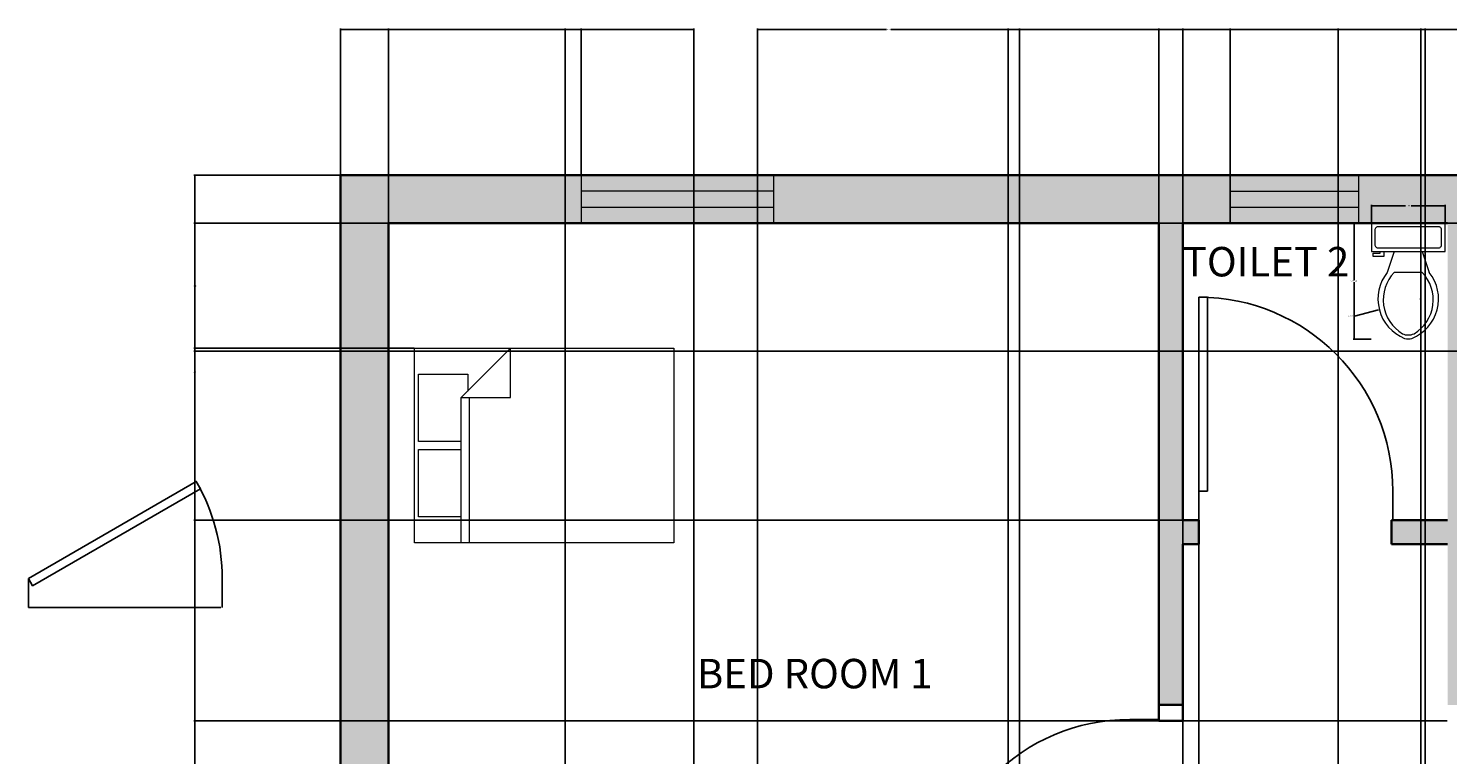
# Model space of a CAD drawing. Units: inches. Extents: x 1839 to 2285, y 722 to 1311.
# Tile 6 of 7: x 1839 to 2105, y 1175 to 1311. Entities that reach past the tile are written whole.
import ezdxf

# ---------------------------------------------------------------- set-up
doc = ezdxf.new("R2010")
doc.units = ezdxf.units.IN
for name, color, linetype, lineweight in [('A-ANNO-DIMS', 2, 'Continuous', 18), ('A-AREA-IDEN', 7, 'Continuous', 18), ('A-DOOR', 3, 'Continuous', 25), ('A-FLOR-FIXT', 9, 'Continuous', 18), ('A-FURN', 8, 'Continuous', 18), ('A-GLAZ', 4, 'Continuous', 18), ('A-GLAZ-PATT', 9, 'Continuous', 13), ('A-WALL', 7, 'Continuous', 35)]:
    doc.layers.add(name, color=color, linetype=linetype, lineweight=lineweight)
doc.layers.add('A-WALL-PATT', color=18, linetype='Continuous', lineweight=13, true_color=0x000000)
doc.styles.get("Standard").update_dxf_attribs({"font": 'arial.ttf'})
doc.dimstyles.get("Standard").update_dxf_attribs({"dimtxt": 0.18, "dimasz": 0.18, "dimexe": 0.18, "dimexo": 0.0625, "dimgap": 0.09, "dimtad": 0, "dimtih": 1, "dimtoh": 1, "dimdec": 4, "dimzin": 0, "dimdsep": 46, "dimtxsty": 'Standard', "dimcen": 0.09, "dimadec": 0, "dimazin": 0, "dimtfac": 1, "dimtdec": 4, "dimtofl": 0, "dimtmove": 0, "dimatfit": 3, "dimfxl": 1, "dimtolj": 1, "dimtzin": 0, "dimarcsym": 0})

# ---------------------------------------------------------------- blocks, each defined once
blk = doc.blocks.new('*U2')
for p, q in [((0, 0), (0, -6)), ((40, 0), (40, -6))]:
    blk.add_line(p, q)
blk.add_lwpolyline([(0, 0), (34.64, 20), (35.52, 18.48), (0.87, -1.52)], close=True)
blk.add_arc((0, 0), 40, 0, 30)
blk = doc.blocks.new('*U4')
for p, q in [((0, 0), (0, -6)), ((40, 0), (40, -6))]:
    blk.add_line(p, q)
blk.add_lwpolyline([(0, 0), (0, 40), (1.75, 40), (1.75, 0)], close=True)
blk.add_arc((0, 0), 40, 0, 90)
blk = doc.blocks.new('Toilet - top')
for p, q in [((9.5, -6), (9.5, -2)), ((-8, -8.5), (-8, -8)), ((-7, -8), (-7, -9.5)), ((-4, -8), (-6, -14)), ((4, -8), (6, -14)), ((-10, -8.5), (-8, -8.5)), ((-10, -9.5), (-10, -8.5)), ((-7, -9.5), (-10, -9.5)), ((4, -14), (-4, -14))]:
    blk.add_line(p, q)
blk.add_lwpolyline([(10.5, -8), (10.5, 0), (-10.5, 0), (-10.5, -8)], close=True)
for points in [[(-9.5, -2), (-9.5, -6)], [(8.5, -1), (-8.5, -1)], [(-8.5, -7), (8.5, -7)]]:
    blk.add_lwpolyline(points)
for centre, radius, start, end in [((-8.62, -1.88), 0.884, 81.8699, 188.1301), ((8.62, -1.88), 0.884, 351.8699, 98.1301), ((-8.62, -6.12), 0.884, 171.8699, 278.1301), ((8.62, -6.12), 0.884, 261.8699, 8.1301), ((3.52, -21.58), 12.17, 141.4691, 247.9714), ((4.2, -21.82), 11.33, 136.3677, 238.9468), ((-3.52, -21.58), 12.17, 292.0284, 38.5307), ((-4.2, -21.82), 11.33, 301.053, 43.6321), ((0, -27.88), 4, 245.7318, 294.2682), ((0, -29), 4, 254.8605, 285.1395)]:
    blk.add_arc(centre, radius, start, end)
blk = doc.blocks.new('Bed - Queen')
for p, q in [((0, -80.00003), (0, 0)), ((0, 0), (59.99999, 0)), ((59.99999, 0), (59.99999, -80.00003)), ((7.99999, -1.2), (28.79998, -1.2)), ((7.99999, -14.4), (7.99999, -1.2)), ((28.79998, -1.2), (28.79998, -14.4)), ((31.19999, -1.2), (51.99999, -1.2)), ((31.19999, -14.4), (31.19999, -1.2)), ((51.99999, -1.2), (51.99999, -16.4)), ((0, -14.4), (44.8, -14.4)), ((44.8, -16.8), (0, -16.8)), ((59.99999, -29.6), (44.8, -14.4)), ((44.8, -14.4), (44.8, -29.6)), ((51.99999, -16.4), (46.79936, -16.4)), ((44.8, -29.6), (59.99999, -29.6)), ((59.99999, -80.00003), (0, -80.00003))]:
    blk.add_line(p, q)
blk = doc.blocks.new('WIN-36x9')
for p, q in [((0, 9), (0, 0)), ((36, 9), (0, 9)), ((36, 0), (36, 9)), ((36, 6), (0, 6)), ((0, 3), (36, 3)), ((0, 0), (36, 0))]:
    blk.add_line(p, q)
blk = doc.blocks.new('WIN-24x9')
for p, q in [((3, 0), (3, 24)), ((6, 0), (6, 24))]:
    blk.add_line(p, q)
blk.add_lwpolyline([(0, 24), (0, 0), (9, 0), (9, 24)], close=True)
blk = doc.blocks.new('*D23')
at = {"layer": 'A-ANNO-DIMS', "color": 0, "lineweight": -2, "transparency": 16777216}
for p, q in [((2090.38, 1274.33), (2087.01, 1274.33)), ((2087.19, 1274.15), (2087.19, 1263.69)), ((2087.19, 1252.87), (2087.19, 1263.33)), ((2090.38, 1252.69), (2087.01, 1252.69))]:
    blk.add_line(p, q, dxfattribs=at)
at = {"layer": 'A-ANNO-DIMS', "color": 0, "transparency": 16777216}
for points in [[(2087.16, 1274.15), (2087.22, 1274.15), (2087.19, 1274.33)], [(2087.16, 1252.87), (2087.22, 1252.87), (2087.19, 1252.69)]]:
    blk.add_solid(points, dxfattribs=at)
at = {"layer": 'Defpoints', "color": 0, "transparency": 16777216}
for p in [(2087.19, 1274.33), (2090.44, 1274.33), (2090.44, 1252.69)]:
    blk.add_point(p, dxfattribs=at)
at = {"layer": 'A-ANNO-DIMS', "color": 0, "transparency": 16777216, "insert": (2087.19, 1263.51), "char_height": 0.18, "attachment_point": 5}
blk.add_mtext('\\A1;WC 22 TYP.', dxfattribs=at)
blk = doc.blocks.new('*D24')
at = {"layer": 'A-ANNO-DIMS', "color": 0, "lineweight": -2, "transparency": 16777216}
for p, q in [((2090.44, 1274.39), (2090.44, 1277.76)), ((2090.62, 1277.58), (2096.8, 1277.58)), ((2104.01, 1277.58), (2097.84, 1277.58)), ((2104.19, 1274.39), (2104.19, 1277.76))]:
    blk.add_line(p, q, dxfattribs=at)
at = {"layer": 'A-ANNO-DIMS', "color": 0, "transparency": 16777216}
for points in [[(2090.62, 1277.61), (2090.62, 1277.55), (2090.44, 1277.58)], [(2104.01, 1277.61), (2104.01, 1277.55), (2104.19, 1277.58)]]:
    blk.add_solid(points, dxfattribs=at)
at = {"layer": 'Defpoints', "color": 0, "transparency": 16777216}
for p in [(2104.19, 1277.58), (2090.44, 1274.33), (2104.19, 1274.33)]:
    blk.add_point(p, dxfattribs=at)
at = {"layer": 'A-ANNO-DIMS', "color": 0, "transparency": 16777216, "insert": (2097.32, 1277.58), "char_height": 0.18, "attachment_point": 5}
blk.add_mtext('\\A1;14 TYP.', dxfattribs=at)
blk = doc.blocks.new('*D42')
at = {"layer": 'A-ANNO-DIMS', "color": 0, "lineweight": -2, "transparency": 16777216}
for p, q in [((1897.61, 1283.33), (1870.25, 1283.33)), ((1870.43, 1283.15), (1870.43, 1043.51)), ((1870.43, 803.51), (1870.43, 1043.15)), ((1897.61, 803.33), (1870.25, 803.33))]:
    blk.add_line(p, q, dxfattribs=at)
at = {"layer": 'A-ANNO-DIMS', "color": 0, "transparency": 16777216}
for points in [[(1870.4, 1283.15), (1870.46, 1283.15), (1870.43, 1283.33)], [(1870.4, 803.51), (1870.46, 803.51), (1870.43, 803.33)]]:
    blk.add_solid(points, dxfattribs=at)
at = {"layer": 'Defpoints', "color": 0, "transparency": 16777216}
for p in [(1870.43, 1283.33), (1897.68, 1283.33), (1897.68, 803.33)]:
    blk.add_point(p, dxfattribs=at)
at = {"layer": 'A-ANNO-DIMS', "color": 0, "transparency": 16777216, "insert": (1870.43, 1043.33), "char_height": 0.18, "attachment_point": 5}
blk.add_mtext('\\A1;480', dxfattribs=at)
blk = doc.blocks.new('*D47')
at = {"layer": 'A-ANNO-DIMS', "color": 0, "lineweight": -2, "transparency": 16777216}
for p, q in [((2055.11, 1274.33), (1870.25, 1274.33)), ((1870.43, 1274.15), (1870.43, 1246.76)), ((1870.43, 1219.01), (1870.43, 1246.4)), ((2055.11, 1218.83), (1870.25, 1218.83))]:
    blk.add_line(p, q, dxfattribs=at)
at = {"layer": 'A-ANNO-DIMS', "color": 0, "transparency": 16777216}
for points in [[(1870.4, 1274.15), (1870.46, 1274.15), (1870.43, 1274.33)], [(1870.4, 1219.01), (1870.46, 1219.01), (1870.43, 1218.83)]]:
    blk.add_solid(points, dxfattribs=at)
at = {"layer": 'Defpoints', "color": 0, "transparency": 16777216}
for p in [(1870.43, 1274.33), (2055.18, 1274.33), (2055.18, 1218.83)]:
    blk.add_point(p, dxfattribs=at)
at = {"layer": 'A-ANNO-DIMS', "color": 0, "transparency": 16777216, "insert": (1870.43, 1246.58), "char_height": 0.18, "attachment_point": 5}
blk.add_mtext('\\A1;55.5', dxfattribs=at)
blk = doc.blocks.new('*D53')
at = {"layer": 'A-ANNO-DIMS', "color": 0, "lineweight": -2, "transparency": 16777216}
for p, q in [((2099.66, 1017.89), (2099.66, 1310.76)), ((2099.84, 1310.58), (2129.54, 1310.58)), ((2160, 1310.58), (2130.3, 1310.58)), ((2160.18, 1017.89), (2160.18, 1310.76))]:
    blk.add_line(p, q, dxfattribs=at)
at = {"layer": 'A-ANNO-DIMS', "color": 0, "transparency": 16777216}
for points in [[(2099.84, 1310.61), (2099.84, 1310.55), (2099.66, 1310.58)], [(2160, 1310.61), (2160, 1310.55), (2160.18, 1310.58)]]:
    blk.add_solid(points, dxfattribs=at)
at = {"layer": 'Defpoints', "color": 0, "transparency": 16777216}
for p in [(2160.18, 1310.58), (2099.66, 1017.83), (2160.18, 1017.83)]:
    blk.add_point(p, dxfattribs=at)
at = {"layer": 'A-ANNO-DIMS', "color": 0, "transparency": 16777216, "insert": (2129.92, 1310.58), "char_height": 0.18, "attachment_point": 5}
blk.add_mtext('\\A1;60.51', dxfattribs=at)
blk = doc.blocks.new('*D55')
at = {"layer": 'A-ANNO-DIMS', "color": 0, "lineweight": -2, "transparency": 16777216}
for p, q in [((2022.5, 812.39), (2022.5, 1310.76)), ((2022.68, 1310.58), (2061.29, 1310.58)), ((2100.32, 1310.58), (2061.72, 1310.58)), ((2100.5, 812.39), (2100.5, 1310.76))]:
    blk.add_line(p, q, dxfattribs=at)
at = {"layer": 'A-ANNO-DIMS', "color": 0, "transparency": 16777216}
for points in [[(2022.68, 1310.61), (2022.68, 1310.55), (2022.5, 1310.58)], [(2100.32, 1310.61), (2100.32, 1310.55), (2100.5, 1310.58)]]:
    blk.add_solid(points, dxfattribs=at)
at = {"layer": 'Defpoints', "color": 0, "transparency": 16777216}
for p in [(2100.5, 1310.58), (2022.5, 812.33), (2100.5, 812.33)]:
    blk.add_point(p, dxfattribs=at)
at = {"layer": 'A-ANNO-DIMS', "color": 0, "transparency": 16777216, "insert": (2061.5, 1310.58), "char_height": 0.18, "attachment_point": 5}
blk.add_mtext('\\A1;78', dxfattribs=at)
blk = doc.blocks.new('*D59')
at = {"layer": 'A-ANNO-DIMS', "color": 0, "lineweight": -2, "transparency": 16777216}
for p, q in [((2024.66, 1017.89), (2024.66, 1310.76)), ((2024.84, 1310.58), (2054.04, 1310.58)), ((2084.02, 1310.58), (2054.82, 1310.58)), ((2084.2, 1017.89), (2084.2, 1310.76))]:
    blk.add_line(p, q, dxfattribs=at)
at = {"layer": 'A-ANNO-DIMS', "color": 0, "transparency": 16777216}
for points in [[(2024.84, 1310.61), (2024.84, 1310.55), (2024.66, 1310.58)], [(2084.02, 1310.61), (2084.02, 1310.55), (2084.2, 1310.58)]]:
    blk.add_solid(points, dxfattribs=at)
at = {"layer": 'Defpoints', "color": 0, "transparency": 16777216}
for p in [(2084.2, 1310.58), (2024.66, 1017.83), (2084.2, 1017.83)]:
    blk.add_point(p, dxfattribs=at)
at = {"layer": 'A-ANNO-DIMS', "color": 0, "transparency": 16777216, "insert": (2054.43, 1310.58), "char_height": 0.18, "attachment_point": 5}
blk.add_mtext('\\A1;59.53', dxfattribs=at)
blk = doc.blocks.new('*D60')
at = {"layer": 'A-ANNO-DIMS', "color": 0, "lineweight": -2, "transparency": 16777216}
for p, q in [((1897.68, 1283.39), (1897.68, 1310.76)), ((1897.86, 1310.58), (1919.95, 1310.58)), ((1942.5, 1310.58), (1920.4, 1310.58)), ((1942.68, 1283.39), (1942.68, 1310.76))]:
    blk.add_line(p, q, dxfattribs=at)
at = {"layer": 'A-ANNO-DIMS', "color": 0, "transparency": 16777216}
for points in [[(1897.86, 1310.61), (1897.86, 1310.55), (1897.68, 1310.58)], [(1942.5, 1310.61), (1942.5, 1310.55), (1942.68, 1310.58)]]:
    blk.add_solid(points, dxfattribs=at)
at = {"layer": 'Defpoints', "color": 0, "transparency": 16777216}
for p in [(1942.68, 1310.58), (1897.68, 1283.33), (1942.68, 1283.33)]:
    blk.add_point(p, dxfattribs=at)
at = {"layer": 'A-ANNO-DIMS', "color": 0, "transparency": 16777216, "insert": (1920.18, 1310.58), "char_height": 0.18, "attachment_point": 5}
blk.add_mtext('\\A1;45', dxfattribs=at)
blk = doc.blocks.new('*D66')
at = {"layer": 'A-ANNO-DIMS', "color": 0, "lineweight": -2, "transparency": 16777216}
for p, q in [((1975.68, 1017.89), (1975.68, 1310.76)), ((1975.86, 1310.58), (1999.77, 1310.58)), ((2024.48, 1310.58), (2000.57, 1310.58)), ((2024.66, 1017.89), (2024.66, 1310.76))]:
    blk.add_line(p, q, dxfattribs=at)
at = {"layer": 'A-ANNO-DIMS', "color": 0, "transparency": 16777216}
for points in [[(1975.86, 1310.61), (1975.86, 1310.55), (1975.68, 1310.58)], [(2024.48, 1310.61), (2024.48, 1310.55), (2024.66, 1310.58)]]:
    blk.add_solid(points, dxfattribs=at)
at = {"layer": 'Defpoints', "color": 0, "transparency": 16777216}
for p in [(2024.66, 1310.58), (1975.68, 1017.83), (2024.66, 1017.83)]:
    blk.add_point(p, dxfattribs=at)
at = {"layer": 'A-ANNO-DIMS', "color": 0, "transparency": 16777216, "insert": (2000.17, 1310.58), "char_height": 0.18, "attachment_point": 5}
blk.add_mtext('\\A1;48.99', dxfattribs=at)
blk = doc.blocks.new('*D69')
at = {"layer": 'A-ANNO-DIMS', "color": 0, "lineweight": -2, "transparency": 16777216}
for p, q in [((2055.18, 1274.39), (2055.18, 1310.76)), ((2055.36, 1310.58), (2059.22, 1310.58)), ((2063.87, 1310.58), (2060.01, 1310.58)), ((2064.05, 1274.39), (2064.05, 1310.76))]:
    blk.add_line(p, q, dxfattribs=at)
at = {"layer": 'A-ANNO-DIMS', "color": 0, "transparency": 16777216}
for points in [[(2055.36, 1310.61), (2055.36, 1310.55), (2055.18, 1310.58)], [(2063.87, 1310.61), (2063.87, 1310.55), (2064.05, 1310.58)]]:
    blk.add_solid(points, dxfattribs=at)
at = {"layer": 'Defpoints', "color": 0, "transparency": 16777216}
for p in [(2064.05, 1310.58), (2055.18, 1274.33), (2064.05, 1274.33)]:
    blk.add_point(p, dxfattribs=at)
at = {"layer": 'A-ANNO-DIMS', "color": 0, "transparency": 16777216, "insert": (2059.61, 1310.58), "char_height": 0.18, "attachment_point": 5}
blk.add_mtext('\\A1;8.874', dxfattribs=at)
blk = doc.blocks.new('*D70')
at = {"layer": 'A-ANNO-DIMS', "color": 0, "lineweight": -2, "transparency": 16777216}
for p, q in [((2104.61, 1181.33), (1870.25, 1181.33)), ((1870.43, 1181.15), (1870.43, 1163.51)), ((1870.43, 1145.51), (1870.43, 1163.15)), ((2104.61, 1145.33), (1870.25, 1145.33))]:
    blk.add_line(p, q, dxfattribs=at)
at = {"layer": 'A-ANNO-DIMS', "color": 0, "transparency": 16777216}
for points in [[(1870.4, 1181.15), (1870.46, 1181.15), (1870.43, 1181.33)], [(1870.4, 1145.51), (1870.46, 1145.51), (1870.43, 1145.33)]]:
    blk.add_solid(points, dxfattribs=at)
at = {"layer": 'Defpoints', "color": 0, "transparency": 16777216}
for p in [(1870.43, 1181.33), (2104.68, 1181.33), (2104.68, 1145.33)]:
    blk.add_point(p, dxfattribs=at)
at = {"layer": 'A-ANNO-DIMS', "color": 0, "transparency": 16777216, "insert": (1870.43, 1163.33), "char_height": 0.18, "attachment_point": 5}
blk.add_mtext('\\A1;36', dxfattribs=at)
blk = doc.blocks.new('*D72')
at = {"layer": 'A-ANNO-DIMS', "color": 0, "lineweight": -2, "transparency": 16777216}
for p, q in [((2050.68, 1274.39), (2050.68, 1310.76)), ((2050.86, 1310.58), (2052.67, 1310.58)), ((2055, 1310.58), (2053.19, 1310.58)), ((2055.18, 1274.39), (2055.18, 1310.76))]:
    blk.add_line(p, q, dxfattribs=at)
at = {"layer": 'A-ANNO-DIMS', "color": 0, "transparency": 16777216}
for points in [[(2050.86, 1310.61), (2050.86, 1310.55), (2050.68, 1310.58)], [(2055, 1310.61), (2055, 1310.55), (2055.18, 1310.58)]]:
    blk.add_solid(points, dxfattribs=at)
at = {"layer": 'Defpoints', "color": 0, "transparency": 16777216}
for p in [(2055.18, 1310.58), (2050.68, 1274.33), (2055.18, 1274.33)]:
    blk.add_point(p, dxfattribs=at)
at = {"layer": 'A-ANNO-DIMS', "color": 0, "transparency": 16777216, "insert": (2052.93, 1310.58), "char_height": 0.18, "attachment_point": 5}
blk.add_mtext('\\A1;4.5', dxfattribs=at)
blk = doc.blocks.new('*D73')
at = {"layer": 'A-ANNO-DIMS', "color": 0, "lineweight": -2, "transparency": 16777216}
for p, q in [((1906.68, 1150.79), (1906.68, 1310.76)), ((1906.86, 1310.58), (1934.8, 1310.58)), ((1963.54, 1310.58), (1935.59, 1310.58)), ((1963.72, 1150.79), (1963.72, 1310.76))]:
    blk.add_line(p, q, dxfattribs=at)
at = {"layer": 'A-ANNO-DIMS', "color": 0, "transparency": 16777216}
for points in [[(1906.86, 1310.61), (1906.86, 1310.55), (1906.68, 1310.58)], [(1963.54, 1310.61), (1963.54, 1310.55), (1963.72, 1310.58)]]:
    blk.add_solid(points, dxfattribs=at)
at = {"layer": 'Defpoints', "color": 0, "transparency": 16777216}
for p in [(1963.72, 1310.58), (1906.68, 1150.73), (1963.72, 1150.73)]:
    blk.add_point(p, dxfattribs=at)
at = {"layer": 'A-ANNO-DIMS', "color": 0, "transparency": 16777216, "insert": (1935.2, 1310.58), "char_height": 0.18, "attachment_point": 5}
blk.add_mtext('\\A1;57.04', dxfattribs=at)
blk = doc.blocks.new('*D78')
at = {"layer": 'A-ANNO-DIMS', "color": 0, "lineweight": -2, "transparency": 16777216}
for p, q in [((2248.61, 1274.33), (1870.25, 1274.33)), ((1870.43, 1274.15), (1870.43, 1262.56)), ((1870.43, 1250.6), (1870.43, 1262.19)), ((2243.88, 1250.42), (1870.25, 1250.42))]:
    blk.add_line(p, q, dxfattribs=at)
at = {"layer": 'A-ANNO-DIMS', "color": 0, "transparency": 16777216}
for points in [[(1870.4, 1274.15), (1870.46, 1274.15), (1870.43, 1274.33)], [(1870.4, 1250.6), (1870.46, 1250.6), (1870.43, 1250.42)]]:
    blk.add_solid(points, dxfattribs=at)
at = {"layer": 'Defpoints', "color": 0, "transparency": 16777216}
for p in [(2248.68, 1274.33), (1870.43, 1250.42), (2243.94, 1250.42)]:
    blk.add_point(p, dxfattribs=at)
at = {"layer": 'A-ANNO-DIMS', "color": 0, "transparency": 16777216, "insert": (1870.43, 1262.38), "char_height": 0.18, "attachment_point": 5}
blk.add_mtext('\\A1;23.91', dxfattribs=at)
blk = doc.blocks.new('*D79')
at = {"layer": 'A-ANNO-DIMS', "color": 0, "lineweight": -2, "transparency": 16777216}
for p, q in [((1906.61, 1274.33), (1870.25, 1274.33)), ((1870.43, 1274.15), (1870.43, 1262.83)), ((1870.43, 1251.15), (1870.43, 1262.47)), ((1911.48, 1250.97), (1870.25, 1250.97))]:
    blk.add_line(p, q, dxfattribs=at)
at = {"layer": 'A-ANNO-DIMS', "color": 0, "transparency": 16777216}
for points in [[(1870.4, 1274.15), (1870.46, 1274.15), (1870.43, 1274.33)], [(1870.4, 1251.15), (1870.46, 1251.15), (1870.43, 1250.97)]]:
    blk.add_solid(points, dxfattribs=at)
at = {"layer": 'Defpoints', "color": 0, "transparency": 16777216}
for p in [(1906.68, 1274.33), (1870.43, 1250.97), (1911.54, 1250.97)]:
    blk.add_point(p, dxfattribs=at)
at = {"layer": 'A-ANNO-DIMS', "color": 0, "transparency": 16777216, "insert": (1870.43, 1262.65), "char_height": 0.18, "attachment_point": 5}
blk.add_mtext('\\A1;23.36', dxfattribs=at)
blk = doc.blocks.new('*D81')
at = {"layer": 'A-ANNO-DIMS', "color": 0, "lineweight": -2, "transparency": 16777216}
for p, q in [((1906.68, 1013.39), (1906.68, 1310.76)), ((1906.86, 1310.58), (1922.96, 1310.58)), ((1939.5, 1310.58), (1923.4, 1310.58)), ((1939.68, 1013.39), (1939.68, 1310.76))]:
    blk.add_line(p, q, dxfattribs=at)
at = {"layer": 'A-ANNO-DIMS', "color": 0, "transparency": 16777216}
for points in [[(1906.86, 1310.61), (1906.86, 1310.55), (1906.68, 1310.58)], [(1939.5, 1310.61), (1939.5, 1310.55), (1939.68, 1310.58)]]:
    blk.add_solid(points, dxfattribs=at)
at = {"layer": 'Defpoints', "color": 0, "transparency": 16777216}
for p in [(1939.68, 1310.58), (1906.68, 1013.33), (1939.68, 1013.33)]:
    blk.add_point(p, dxfattribs=at)
at = {"layer": 'A-ANNO-DIMS', "color": 0, "transparency": 16777216, "insert": (1923.18, 1310.58), "char_height": 0.18, "attachment_point": 5}
blk.add_mtext('\\A1;33', dxfattribs=at)
blk = doc.blocks.new('*D84')
at = {"layer": 'A-ANNO-DIMS', "color": 0, "lineweight": -2, "transparency": 16777216}
for p, q in [((2055.18, 1218.77), (2055.18, 722.34)), ((2058.18, 1218.77), (2058.18, 722.34)), ((2055.36, 722.52), (2056.53, 722.52)), ((2058, 722.52), (2056.83, 722.52))]:
    blk.add_line(p, q, dxfattribs=at)
at = {"layer": 'A-ANNO-DIMS', "color": 0, "transparency": 16777216}
for points in [[(2055.36, 722.55), (2055.36, 722.49), (2055.18, 722.52)], [(2058, 722.55), (2058, 722.49), (2058.18, 722.52)]]:
    blk.add_solid(points, dxfattribs=at)
at = {"layer": 'Defpoints', "color": 0, "transparency": 16777216}
for p in [(2055.18, 1218.83), (2058.18, 1218.83), (2058.18, 722.52)]:
    blk.add_point(p, dxfattribs=at)
at = {"layer": 'A-ANNO-DIMS', "color": 0, "transparency": 16777216, "insert": (2056.68, 722.52), "char_height": 0.18, "attachment_point": 5}
blk.add_mtext('\\A1;3', dxfattribs=at)
blk = doc.blocks.new('*D91')
at = {"layer": 'A-ANNO-DIMS', "color": 0, "lineweight": -2, "transparency": 16777216}
for p, q in [((2087.29, 1256.96), (2091.74, 1258.13)), ((2099.53, 1260.2), (2099.71, 1260.2)), ((2099.62, 1260.11), (2099.62, 1260.29))]:
    blk.add_line(p, q, dxfattribs=at)
at = {"layer": 'A-ANNO-DIMS', "color": 0, "transparency": 16777216}
blk.add_solid([(2091.73, 1258.16), (2091.75, 1258.1), (2091.91, 1258.17)], dxfattribs=at)
at = {"layer": 'Defpoints', "color": 0, "transparency": 16777216}
for p in [(2091.91, 1258.17), (2099.62, 1260.2)]:
    blk.add_point(p, dxfattribs=at)
at = {"layer": 'A-ANNO-DIMS', "color": 0, "transparency": 16777216, "insert": (2086.61, 1256.96), "char_height": 0.18, "attachment_point": 5}
blk.add_mtext('\\A1;4X R7.968', dxfattribs=at)

msp = doc.modelspace()

# ---------------------------------------------------------------- hatches: boundary and pattern name
at = {"layer": 'A-GLAZ-PATT'}
h = msp.add_hatch(color=256, dxfattribs=at)
h.dxf.hatch_style = 1
h.set_gradient(color1=(0, 0, 255), color2=(255, 255, 0), name='INVCYLINDER')
h.paths.add_polyline_path([(1978.6771, 1283.3314), (1942.6771, 1283.3314), (1942.6771, 1280.3314), (1978.6771, 1280.3314)])
h.paths.add_polyline_path([(1978.6771, 1280.3314), (1942.6771, 1280.3314), (1942.6771, 1277.3314), (1978.6771, 1277.3314)])
h.paths.add_polyline_path([(1978.6771, 1277.3314), (1942.6771, 1277.3314), (1942.6771, 1274.3314), (1978.6771, 1274.3314)])
h = msp.add_hatch(color=256, dxfattribs=at)
h.dxf.hatch_style = 1
h.set_gradient(color1=(0, 0, 255), color2=(255, 255, 0), name='INVCYLINDER')
h.paths.add_polyline_path([(2088.0508, 1283.3314), (2064.0508, 1283.3314), (2064.0508, 1280.3314), (2088.0508, 1280.3314)])
h.paths.add_polyline_path([(2088.0508, 1280.3314), (2064.0508, 1280.3314), (2064.0508, 1277.3314), (2088.0508, 1277.3314)])
h.paths.add_polyline_path([(2088.0508, 1277.3314), (2064.0508, 1277.3314), (2064.0508, 1274.3314), (2088.0508, 1274.3314)])
at = {"layer": 'A-WALL-PATT'}
h = msp.add_hatch(color=256, dxfattribs=at)
h.dxf.hatch_style = 1
h.paths.add_polyline_path([(1906.6771, 1274.3314), (1942.6771, 1274.3314), (1942.6771, 1283.3314), (1897.6771, 1283.3314), (1897.6771, 968.2107), (1906.6771, 968.2107), (1906.6771, 1013.3314), (1939.6771, 1013.3314), (1939.6771, 1017.8314), (1906.6771, 1017.8314), (1906.6771, 1137.8314), (2050.6771, 1137.8314), (2050.6771, 1142.3314), (1906.6771, 1142.3314)])
h.paths.add_polyline_path([(2064.0508, 1283.3314), (1978.6771, 1283.3314), (1978.6771, 1274.3314), (2050.6771, 1274.3314), (2050.6771, 1184.3314), (2055.1771, 1184.3314), (2055.1771, 1214.3314), (2058.1771, 1214.3314), (2058.1771, 1218.8314), (2055.1771, 1218.8314), (2055.1771, 1274.3314), (2064.0508, 1274.3314)])
h.paths.add_polyline_path([(2182.6416, 1283.3314), (2088.0508, 1283.3314), (2088.0508, 1274.3314), (2104.6771, 1274.3314), (2104.6771, 1218.8314), (2094.1771, 1218.8314), (2094.1771, 1214.3314), (2104.6771, 1214.3314), (2104.6771, 1184.3314), (2109.1771, 1184.3314), (2109.1771, 1274.3314), (2182.6416, 1274.3314)])
h.paths.add_polyline_path([(2257.6771, 1283.3314), (2218.6416, 1283.3314), (2218.6416, 1274.3314), (2248.6771, 1274.3314), (2248.6771, 1142.3314), (2186.4004, 1142.3314), (2109.1771, 1142.3314), (2109.1771, 1137.8314), (2248.6771, 1137.8314), (2248.6771, 1094.9086), (2257.6771, 1094.9086)])
h.paths.add_polyline_path([(2257.6771, 1058.9086), (2248.6771, 1058.9086), (2248.6771, 1017.8314), (2160.1771, 1017.8314), (2160.1771, 939.8314), (2164.6771, 939.8314), (2164.6771, 1013.3314), (2248.6771, 1013.3314), (2248.6771, 977.3314), (2248.6771, 950.4862), (2257.6771, 950.4862)])
h.paths.add_polyline_path([(2257.6771, 893.3314), (2248.6771, 893.3314), (2248.6771, 850.1143), (2190.4862, 850.1143), (2190.4862, 845.6143), (2248.6771, 845.6143), (2248.6771, 812.3314), (2100.5038, 812.3314), (2100.5038, 803.3314), (2257.6771, 803.3314)])
h.paths.add_polyline_path([(2257.6771, 926.4862), (2248.6771, 926.4862), (2248.6771, 897.8314), (2141.6642, 897.8314), (2141.6642, 893.3314), (2145.5038, 893.3314), (2145.5038, 812.3314), (2147.5038, 812.3314), (2147.5038, 845.6143), (2153.9854, 845.6143), (2153.9854, 850.1143), (2147.5038, 850.1143), (2147.5038, 893.3314), (2248.6771, 893.3314), (2257.6771, 893.3314)])
h.paths.add_polyline_path([(1906.6771, 893.3314), (1897.6771, 893.3314), (1897.6771, 803.3314), (2022.5038, 803.3314), (2022.5038, 812.3314), (1906.6771, 812.3314)])
h.paths.add_polyline_path([(2031.4676, 897.8314), (1981.6771, 897.8314), (1981.6771, 1013.3314), (2024.6642, 1013.3314), (2024.6642, 1017.8314), (1975.6771, 1017.8314), (1975.6771, 1013.3314), (1978.6771, 1013.3314), (1978.6771, 897.8314), (1906.6771, 897.8314), (1906.6771, 932.2107), (1897.6771, 932.2107), (1897.6771, 893.3314), (1906.6771, 893.3314), (2031.4676, 893.3314)])
h.paths.add_polyline_path([(2099.6642, 1017.8314), (2096.6642, 1017.8314), (2084.1956, 1017.8314), (2084.1956, 1013.3314), (2096.6642, 1013.3314), (2096.6642, 897.8314), (2085.6129, 897.8314), (2085.6129, 893.3314), (2102.6642, 893.3314), (2102.6642, 897.8314), (2099.6642, 897.8314)])

# ---------------------------------------------------------------- linework, layer by layer
at = {"layer": 'A-DOOR'}
msp.add_line((1839.3305, 1202.5199), (1875.3305, 1202.5199), dxfattribs=at)
at = {"layer": 'A-WALL'}
for p, q in [((1906.6771, 1274.3314), (2050.6771, 1274.3314)), ((1906.6771, 1142.3314), (1906.6771, 1274.3314)), ((2050.6771, 1181.3314), (2050.6771, 1274.3314)), ((2055.1771, 1218.8314), (2055.1771, 1274.3314)), ((2055.1771, 1274.3314), (2104.6771, 1274.3314)), ((2055.1771, 1218.8314), (2058.1771, 1218.8314)), ((2058.1771, 1214.3314), (2058.1771, 1218.8314)), ((2094.1771, 1214.3314), (2094.1771, 1218.8314)), ((2094.1771, 1218.8314), (2104.6771, 1218.8314)), ((2055.1771, 1214.3314), (2058.1771, 1214.3314)), ((2055.1771, 1181.3314), (2055.1771, 1214.3314)), ((2094.1771, 1214.3314), (2104.6771, 1214.3314)), ((2050.6771, 1184.3314), (2055.1771, 1184.3314)), ((2050.6771, 1181.3314), (2055.1771, 1181.3314))]:
    msp.add_line(p, q, dxfattribs=at)
msp.add_lwpolyline([(2022.5038, 803.3314), (1897.6771, 803.3314), (1897.6771, 1283.3314), (2257.6771, 1283.3314), (2257.6771, 803.3314), (2100.5038, 803.3314)], dxfattribs=at)

# ---------------------------------------------------------------- block references
at = {"layer": 'A-DOOR', "xscale": 0.9062393225401889, "yscale": 0.9062393225401889, "zscale": 0.9062393225401889}
for name, p in [('*U4', (2058.1771, 1224.2689)), ('*U2', (1839.3305, 1207.9573))]:
    msp.add_blockref(name, p, dxfattribs=at)
at = {"layer": 'A-DOOR', "xscale": 0.9062393225401889, "yscale": 0.9062393225401889, "zscale": 0.9062393225401889, "rotation": 90}
msp.add_blockref('*U4', (2045.2397, 1145.3314), dxfattribs=at)
at = {"layer": 'A-FLOR-FIXT', "xscale": 0.6548161329715463, "yscale": 0.6548161329715463, "zscale": 0.6548161329715463}
msp.add_blockref('Toilet - top', (2097.3161, 1274.3314), dxfattribs=at)
at = {"layer": 'A-FURN', "xscale": 0.6058629736700599, "yscale": 0.6058629736700599, "zscale": 0.6058629736700599, "rotation": 90}
msp.add_blockref('Bed - Queen', (1911.5419, 1214.6177), dxfattribs=at)
at = {"layer": 'A-GLAZ'}
msp.add_blockref('WIN-36x9', (1942.6775, 1274.331), dxfattribs=at)
at = {"layer": 'A-GLAZ', "rotation": 270.0000000000008}
msp.add_blockref('WIN-24x9', (2064.0506, 1283.3315), dxfattribs=at)

# ---------------------------------------------------------------- texts
at = {"layer": 'A-AREA-IDEN'}
for s, height, p in [('TOILET 2 ', 5.50379, (2055.1771, 1264.4057)), ('BED ROOM 1 ', 5.503795, (1964.3239, 1187.4184))]:
    msp.add_text(s, height=height, dxfattribs=at).set_placement(p)

# ---------------------------------------------------------------- dimensions: what is measured, and where the dimension line sits
at = {"layer": 'A-ANNO-DIMS'}
for base, p1, p2, override, picture, middle in [((1942.6771, 1310.5814), (1897.6771, 1283.3314), (1942.6771, 1283.3314), {"dimdec": 0, "dimlfac": 1, "dimrnd": 0, "dimzin": 0, "dimdsep": 46, "dimlunit": 2}, '*D60', (1920.1771, 1310.5814)), ((1963.7186, 1310.5814), (1906.6771, 1150.7318), (1963.7186, 1150.7318), {"dimdec": 2, "dimlfac": 1, "dimrnd": 0, "dimzin": 0, "dimdsep": 46, "dimlunit": 2}, '*D73', (1935.1978, 1310.5814)), ((1939.6771, 1310.5814), (1906.6771, 1013.3314), (1939.6771, 1013.3314), {"dimdec": 0, "dimlfac": 1, "dimrnd": 0, "dimzin": 0, "dimdsep": 46, "dimlunit": 2}, '*D81', (1923.1771, 1310.5814)), ((2024.6642, 1310.5814), (1975.6771, 1017.8314), (2024.6642, 1017.8314), {"dimdec": 2, "dimlfac": 1, "dimrnd": 0, "dimzin": 0, "dimdsep": 46, "dimlunit": 2}, '*D66', (2000.1706, 1310.5814)), ((2100.5038, 1310.5814), (2022.5038, 812.3314), (2100.5038, 812.3314), {"dimdec": 0, "dimlfac": 1, "dimrnd": 0, "dimzin": 0, "dimdsep": 46, "dimlunit": 2}, '*D55', (2061.5038, 1310.5814)), ((2084.1956, 1310.5814), (2024.6642, 1017.8314), (2084.1956, 1017.8314), {"dimdec": 2, "dimlfac": 1, "dimrnd": 0, "dimzin": 0, "dimdsep": 46, "dimlunit": 2}, '*D59', (2054.4299, 1310.5814)), ((2055.1771, 1310.5814), (2050.6771, 1274.3314), (2055.1771, 1274.3314), {"dimdec": 1, "dimlfac": 1, "dimrnd": 0, "dimzin": 0, "dimdsep": 46, "dimlunit": 2}, '*D72', (2052.9271, 1310.5814)), ((2064.0508, 1310.5814), (2055.1771, 1274.3314), (2064.0508, 1274.3314), {"dimdec": 3, "dimlfac": 1, "dimrnd": 0, "dimzin": 0, "dimdsep": 46, "dimlunit": 2}, '*D69', (2059.614, 1310.5814)), ((2160.1771, 1310.5814), (2099.6642, 1017.8314), (2160.1771, 1017.8314), {"dimdec": 2, "dimlfac": 1, "dimrnd": 0, "dimzin": 0, "dimdsep": 46, "dimlunit": 2}, '*D53', (2129.9206, 1310.5814)), ((2058.1771, 722.516), (2055.1771, 1218.8314), (2058.1771, 1218.8314), {"dimdec": 0, "dimlfac": 1, "dimrnd": 0, "dimzin": 0, "dimdsep": 46, "dimlunit": 2}, '*D84', (2056.6771, 722.516))]:
    dim = msp.add_linear_dim(base=base, p1=p1, p2=p2, dimstyle='Standard', override=override, dxfattribs=at)
    dim.commit()
    dim.dimension.update_dxf_attribs({"geometry": picture, "text_midpoint": middle})
for base, p1, p2, override, picture, middle in [((1870.4271, 1283.3314), (1897.6771, 803.3314), (1897.6771, 1283.3314), {"dimdec": 0, "dimlfac": 1, "dimrnd": 0, "dimzin": 0, "dimdsep": 46, "dimlunit": 2}, '*D42', (1870.4271, 1043.3314)), ((1870.4271, 1250.4215), (2248.6771, 1274.3314), (2243.9435, 1250.4215), {"dimdec": 2, "dimlfac": 1, "dimrnd": 0, "dimzin": 0, "dimdsep": 46, "dimlunit": 2}, '*D78', (1870.4271, 1262.3765)), ((1870.4271, 1250.9695), (1906.6771, 1274.3314), (1911.5419, 1250.9695), {"dimdec": 2, "dimlfac": 1, "dimrnd": 0, "dimzin": 0, "dimdsep": 46, "dimlunit": 2}, '*D79', (1870.4271, 1262.6505)), ((1870.4271, 1274.3314), (2055.1771, 1218.8314), (2055.1771, 1274.3314), {"dimdec": 1, "dimlfac": 1, "dimrnd": 0, "dimzin": 0, "dimdsep": 46, "dimlunit": 2}, '*D47', (1870.4271, 1246.5814)), ((1870.4271, 1181.3314), (2104.6771, 1145.3314), (2104.6771, 1181.3314), {"dimdec": 0, "dimlfac": 1, "dimrnd": 0, "dimzin": 0, "dimdsep": 46, "dimlunit": 2}, '*D70', (1870.4271, 1163.3314))]:
    dim = msp.add_linear_dim(base=base, p1=p1, p2=p2, angle=90, dimstyle='Standard', override=override, dxfattribs=at)
    dim.commit()
    dim.dimension.update_dxf_attribs({"geometry": picture, "text_midpoint": middle})
dim = msp.add_linear_dim(base=(2104.1916, 1277.5773), p1=(2090.4405, 1274.3314), p2=(2104.1916, 1274.3314), text='<> TYP.', dimstyle='Standard', override={"dimdec": 0, "dimlfac": 1, "dimrnd": 0, "dimzin": 0, "dimdsep": 46, "dimlunit": 2}, dxfattribs=at)
dim.commit()
dim.dimension.update_dxf_attribs({"geometry": '*D24', "text_midpoint": (2097.3161, 1277.5773)})
dim = msp.add_linear_dim(base=(2087.1946, 1274.3314), p1=(2090.4405, 1252.6922), p2=(2090.4405, 1274.3314), angle=90, text='WC <> TYP.', dimstyle='Standard', override={"dimdec": 0, "dimlfac": 1, "dimrnd": 0, "dimzin": 0, "dimdsep": 46, "dimlunit": 2}, dxfattribs=at)
dim.commit()
dim.dimension.update_dxf_attribs({"geometry": '*D23', "text_midpoint": (2087.1946, 1263.5118)})
dim = msp.add_radius_dim(center=(2099.6207, 1260.2002), mpoint=(2091.9139, 1258.175), text='4X <>', dimstyle='Standard', override={"dimdec": 3, "dimlfac": 1, "dimrnd": 0, "dimzin": 0, "dimdsep": 46, "dimlunit": 2}, dxfattribs=at)
dim.commit()
dim.dimension.update_dxf_attribs({"geometry": '*D91', "text_midpoint": (2087.2898, 1256.9599), "dimtype": 164})

doc.saveas('drawing.dxf')
